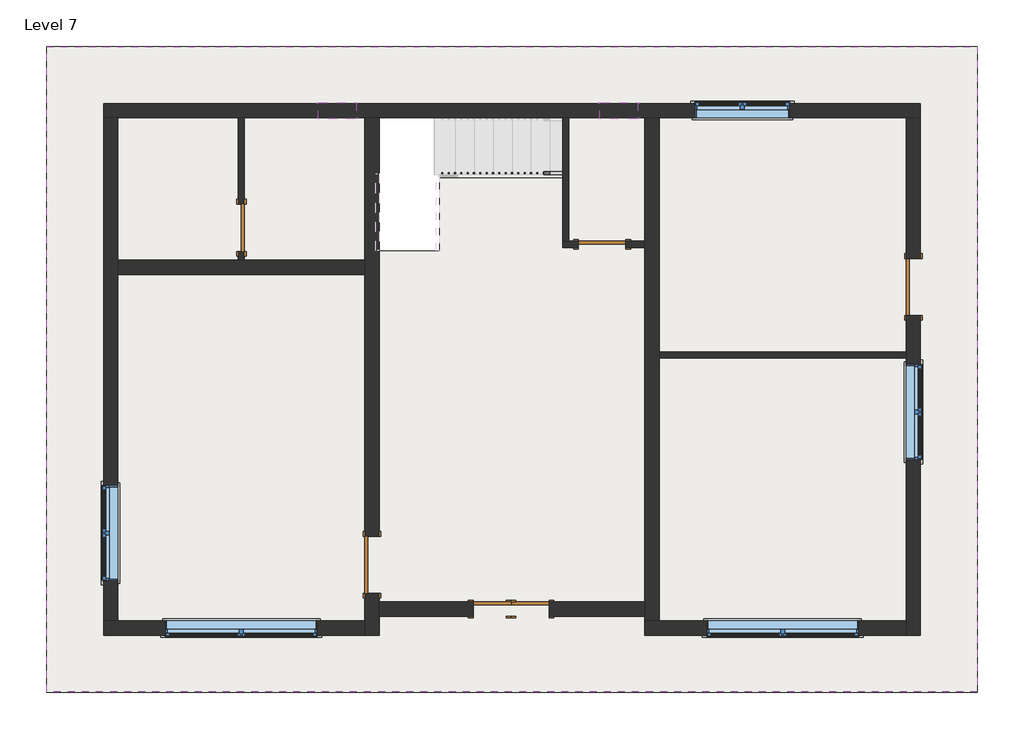
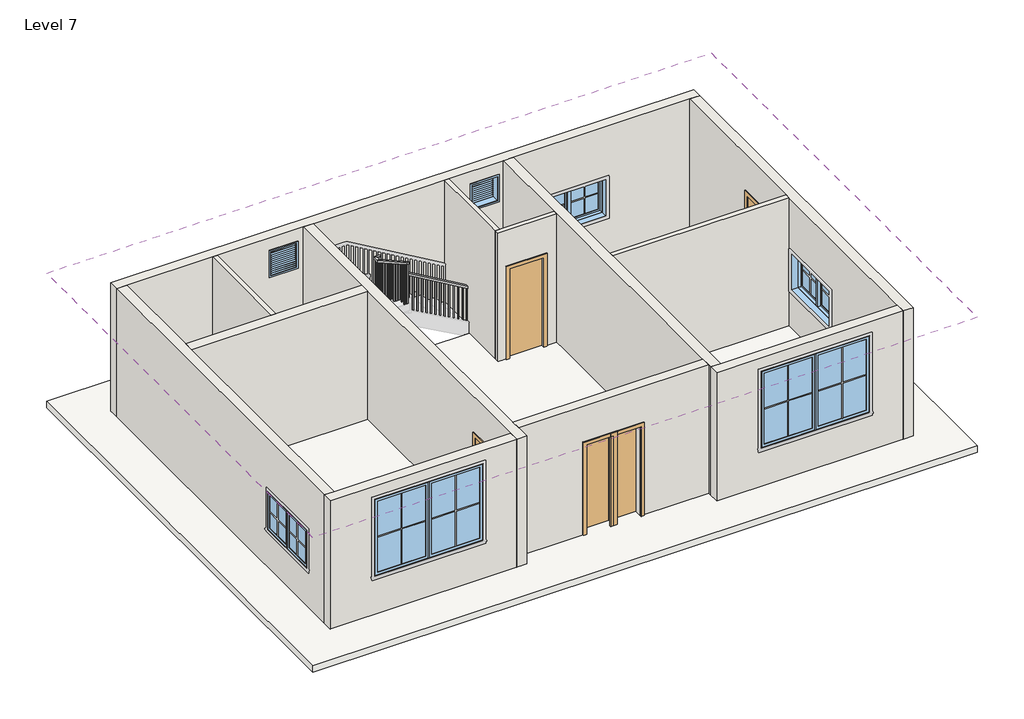
# One storey, part 1 of 2: 13 walls, 7 windows, 6 doors, 2 roofs, 1 railing.
"""IFC4 building model written with IfcOpenShell, lengths in millimetres."""

from ifc_helpers import new_model, si_unit, frame, origin, place, context, project, spatial, polyline, outline, extrude, faceted_brep, transform, mapped, element, save
from components import single_flush_door_2_4a3212df, single_flush_door_2_0d3b4037, door_270f2424, door_aa9e95e7, single_flush_door_3_a90ba1ad, window_casement_double_c1d95f0f, window_casement_double_9ae172a2, window_f2d8fef0

model = new_model("IFC4")

# Units and contexts
model_context = context("Model", 3, world=origin())
ifc_project = project(units=[si_unit("LENGTHUNIT", "METRE", prefix="MILLI")], contexts=[model_context])

# Site, building, storey
site = spatial("IfcSite", under=ifc_project)
building = spatial("IfcBuilding", under=site)
storey = spatial("IfcBuildingStorey", under=building, Name="Level 7", Elevation=19050.0)

# Doors
placement = place(None, origin())
single_flush_door_2_shape = single_flush_door_2_4a3212df(model_context)
element("IfcDoor", 1, ObjectType="Single-Flush : DOOR 2'", at=placement, inside=storey, context=model_context, shape_type="MappedRepresentation", body=[
    mapped(single_flush_door_2_shape, transform((-1572.7415084, -2604.3618005, 19050.0), x_axis=(-1.0, 0.0, 0.0), y_axis=(0.0, -1.0, 0.0), z_axis=(0.0, 0.0, 1.0))),
])
single_flush_door_2_2_shape = single_flush_door_2_0d3b4037(model_context)
element("IfcDoor", 2, ObjectType="Single-Flush : DOOR 2'", at=placement, inside=storey, context=model_context, shape_type="MappedRepresentation", body=[
    mapped(single_flush_door_2_2_shape, transform((-963.1415084, -2604.3618005, 19050.0), x_axis=(1.0, 0.0, 0.0), y_axis=(0.0, 1.0, 0.0), z_axis=(0.0, 0.0, 1.0))),
])
door_shape = door_270f2424(model_context)
element("IfcDoor", 3, ObjectType="Single-Flush : DOOR 2'6\"", at=placement, inside=storey, context=model_context, shape_type="MappedRepresentation", body=[
    mapped(door_shape, transform((-5598.6415084, 3517.0381995, 19050.0), x_axis=(0.0, -1.0, 0.0), y_axis=(1.0, 0.0, 0.0), z_axis=(0.0, 0.0, 1.0))),
])
door_2_shape = door_aa9e95e7(model_context)
element("IfcDoor", 4, ObjectType="Single-Flush : DOOR 2'6\"", at=placement, inside=storey, context=model_context, shape_type="MappedRepresentation", body=[
    mapped(door_2_shape, transform((192.5584916, 3250.3381995, 19050.0), x_axis=(-1.0, 0.0, 0.0), y_axis=(0.0, -1.0, 0.0), z_axis=(0.0, 0.0, 1.0))),
])
single_flush_door_3_shape = single_flush_door_3_a90ba1ad(model_context)
element("IfcDoor", 5, ObjectType="Single-Flush : DOOR 3'", at=placement, inside=storey, context=model_context, shape_type="MappedRepresentation", body=[
    mapped(single_flush_door_3_shape, transform((-3503.1415084, -1893.1618005, 19050.0), x_axis=(0.0, -1.0, 0.0), y_axis=(1.0, 0.0, 0.0), z_axis=(0.0, 0.0, 1.0))),
])
element("IfcDoor", 6, ObjectType="Single-Flush : DOOR 3'", at=placement, inside=storey, context=model_context, shape_type="MappedRepresentation", body=[
    mapped(single_flush_door_3_shape, transform((5183.6584916, 2564.5381995, 19050.0), x_axis=(0.0, -1.0, 0.0), y_axis=(1.0, 0.0, 0.0), z_axis=(0.0, 0.0, 1.0))),
])

# Railing
element("IfcRailing", 7, ObjectType="Handrail - Rectangular", at=placement, inside=storey, context=model_context, shape_type="SolidModel", body=[
    faceted_brep([(-442.4415084, 4368.3146777, 20133.7333333), (-442.4415084, 4368.3146777, 20074.9219871), (-442.4415084, 4419.1146777, 20074.9219871), (-442.4415084, 4419.1146777, 20133.7333333), (-2398.2415084, 4368.3146777, 21274.6166667), (-2449.0415084, 4368.3146777, 21245.4386538), (-2449.0415084, 4419.1146777, 21245.4386538), (-2398.2415084, 4419.1146777, 21274.6166667), (-2398.2415084, 4368.3146777, 21530.7202697), (-2449.0415084, 4368.3146777, 21479.9202697), (-2449.0415084, 4419.1146777, 21479.9202697), (-2398.2415084, 4419.1146777, 21530.7202697), (-2474.4415084, 4368.3146777, 21530.7202697), (-2474.4415084, 4368.3146777, 21479.9202697), (-2525.2415084, 4419.1146777, 21479.9202697), (-2525.2415084, 4419.1146777, 21530.7202697), (-2474.4415084, 4292.1146777, 21530.7202697), (-2474.4415084, 4278.9546266, 21479.9202697), (-2525.2415084, 4278.9546266, 21479.9202697), (-2525.2415084, 4292.1146777, 21530.7202697), (-2474.4415084, 3148.7383287, 22165.7333333), (-2525.2415084, 3148.7383287, 22165.7333333), (-2525.2415084, 3148.7383287, 22107.62445), (-2474.4415084, 3148.7383287, 22107.62445)], [[[0, 1, 2, 3]], [[1, 0, 4, 5]], [[2, 1, 5, 6]], [[3, 2, 6, 7]], [[0, 3, 7, 4]], [[5, 4, 8, 9]], [[6, 5, 9, 10]], [[7, 6, 10, 11]], [[4, 7, 11, 8]], [[9, 8, 12, 13]], [[10, 9, 13, 14]], [[11, 10, 14, 15]], [[8, 11, 15, 12]], [[13, 12, 16, 17]], [[14, 13, 17, 18]], [[15, 14, 18, 19]], [[12, 15, 19, 16]], [[20, 21, 22, 23]], [[17, 16, 20, 23]], [[18, 17, 23, 22]], [[19, 18, 22, 21]], [[16, 19, 21, 20]]]),
    extrude(outline(polyline([(3184.0396777, 22088.1754052), (3184.0396777, 21082.0), (3164.9896777, 21082.0), (3164.9896777, 22098.7554726), (3184.0396777, 22088.1754052)])), frame((-2509.3665084, 0.0, 0.0), z_axis=(1.0, 0.0, 0.0), x_axis=(0.0, 1.0, 0.0)), (0.0, 0.0, 1.0), 19.05),
    extrude(outline(polyline([(3285.6396777, 22031.7483789), (3285.6396777, 21082.0), (3266.5896777, 21082.0), (3266.5896777, 22042.3284463), (3285.6396777, 22031.7483789)])), frame((-2509.3665084, 0.0, 0.0), z_axis=(1.0, 0.0, 0.0), x_axis=(0.0, 1.0, 0.0)), (0.0, 0.0, 1.0), 19.05),
    extrude(outline(polyline([(3387.2396777, 21975.3213526), (3387.2396777, 21082.0), (3368.1896777, 21082.0), (3368.1896777, 21985.9014201), (3387.2396777, 21975.3213526)])), frame((-2509.3665084, 0.0, 0.0), z_axis=(1.0, 0.0, 0.0), x_axis=(0.0, 1.0, 0.0)), (0.0, 0.0, 1.0), 19.05),
    extrude(outline(polyline([(3488.8396777, 21918.8420718), (3488.8396777, 20912.6666667), (3469.7896777, 20912.6666667), (3469.7896777, 21929.4221392), (3488.8396777, 21918.8420718)])), frame((-2509.3665084, 0.0, 0.0), z_axis=(1.0, 0.0, 0.0), x_axis=(0.0, 1.0, 0.0)), (0.0, 0.0, 1.0), 19.05),
    extrude(outline(polyline([(3590.4396777, 21862.4150456), (3590.4396777, 20912.6666667), (3571.3896777, 20912.6666667), (3571.3896777, 21872.995113), (3590.4396777, 21862.4150456)])), frame((-2509.3665084, 0.0, 0.0), z_axis=(1.0, 0.0, 0.0), x_axis=(0.0, 1.0, 0.0)), (0.0, 0.0, 1.0), 19.05),
    extrude(outline(polyline([(3692.0396777, 21805.9880193), (3692.0396777, 20912.6666667), (3672.9896777, 20912.6666667), (3672.9896777, 21816.5680867), (3692.0396777, 21805.9880193)])), frame((-2509.3665084, 0.0, 0.0), z_axis=(1.0, 0.0, 0.0), x_axis=(0.0, 1.0, 0.0)), (0.0, 0.0, 1.0), 19.05),
    extrude(outline(polyline([(3793.6396777, 21749.5087385), (3793.6396777, 20743.3333333), (3774.5896777, 20743.3333333), (3774.5896777, 21760.0888059), (3793.6396777, 21749.5087385)])), frame((-2509.3665084, 0.0, 0.0), z_axis=(1.0, 0.0, 0.0), x_axis=(0.0, 1.0, 0.0)), (0.0, 0.0, 1.0), 19.05),
    extrude(outline(polyline([(3895.2396777, 21693.0817122), (3895.2396777, 20743.3333333), (3876.1896777, 20743.3333333), (3876.1896777, 21703.6617797), (3895.2396777, 21693.0817122)])), frame((-2509.3665084, 0.0, 0.0), z_axis=(1.0, 0.0, 0.0), x_axis=(0.0, 1.0, 0.0)), (0.0, 0.0, 1.0), 19.05),
    extrude(outline(polyline([(3996.8396777, 21636.654686), (3996.8396777, 20743.3333333), (3977.7896777, 20743.3333333), (3977.7896777, 21647.2347534), (3996.8396777, 21636.654686)])), frame((-2509.3665084, 0.0, 0.0), z_axis=(1.0, 0.0, 0.0), x_axis=(0.0, 1.0, 0.0)), (0.0, 0.0, 1.0), 19.05),
    extrude(outline(polyline([(4098.4396777, 21580.1754052), (4098.4396777, 20574.0), (4079.3896777, 20574.0), (4079.3896777, 21590.7554726), (4098.4396777, 21580.1754052)])), frame((-2509.3665084, 0.0, 0.0), z_axis=(1.0, 0.0, 0.0), x_axis=(0.0, 1.0, 0.0)), (0.0, 0.0, 1.0), 19.05),
    extrude(outline(polyline([(4200.0396777, 21523.7483789), (4200.0396777, 20574.0), (4180.9896777, 20574.0), (4180.9896777, 21534.3284463), (4200.0396777, 21523.7483789)])), frame((-2509.3665084, 0.0, 0.0), z_axis=(1.0, 0.0, 0.0), x_axis=(0.0, 1.0, 0.0)), (0.0, 0.0, 1.0), 19.05),
    extrude(outline(polyline([(4301.6396777, 21467.3213526), (4301.6396777, 20574.0), (4282.5896777, 20574.0), (4282.5896777, 21477.9014201), (4301.6396777, 21467.3213526)])), frame((-2509.3665084, 0.0, 0.0), z_axis=(1.0, 0.0, 0.0), x_axis=(0.0, 1.0, 0.0)), (0.0, 0.0, 1.0), 19.05),
    extrude(outline(polyline([(-2464.9165084, 4384.1896777), (-2483.9665084, 4384.1896777), (-2483.9665084, 4403.2396777), (-2464.9165084, 4403.2396777), (-2464.9165084, 4384.1896777)])), frame((0.0, 0.0, 20404.6666667), z_axis=(0.0, 0.0, 1.0), x_axis=(1.0, 0.0, 0.0)), (0.0, 0.0, 1.0), 1075.253603),
    extrude(outline(polyline([(21206.5449038, -2382.3665084), (20235.3333333, -2382.3665084), (20235.3333333, -2363.3165084), (21195.4324038, -2363.3165084), (21206.5449038, -2382.3665084)])), frame((0.0, 4384.1896777, 0.0), z_axis=(0.0, 1.0, 0.0), x_axis=(0.0, 0.0, 1.0)), (0.0, 0.0, 1.0), 19.05),
    extrude(outline(polyline([(21147.2782371, -2280.7665084), (20235.3333333, -2280.7665084), (20235.3333333, -2261.7165084), (21136.1657371, -2261.7165084), (21147.2782371, -2280.7665084)])), frame((0.0, 4384.1896777, 0.0), z_axis=(0.0, 1.0, 0.0), x_axis=(0.0, 0.0, 1.0)), (0.0, 0.0, 1.0), 19.05),
    extrude(outline(polyline([(21088.0115704, -2179.1665084), (20235.3333333, -2179.1665084), (20235.3333333, -2160.1165084), (21076.8990704, -2160.1165084), (21088.0115704, -2179.1665084)])), frame((0.0, 4384.1896777, 0.0), z_axis=(0.0, 1.0, 0.0), x_axis=(0.0, 0.0, 1.0)), (0.0, 0.0, 1.0), 19.05),
    extrude(outline(polyline([(21028.7449038, -2077.5665084), (20066.0, -2077.5665084), (20066.0, -2058.5165084), (21017.6324038, -2058.5165084), (21028.7449038, -2077.5665084)])), frame((0.0, 4384.1896777, 0.0), z_axis=(0.0, 1.0, 0.0), x_axis=(0.0, 0.0, 1.0)), (0.0, 0.0, 1.0), 19.05),
    extrude(outline(polyline([(20969.4782371, -1975.9665084), (20066.0, -1975.9665084), (20066.0, -1956.9165084), (20958.3657371, -1956.9165084), (20969.4782371, -1975.9665084)])), frame((0.0, 4384.1896777, 0.0), z_axis=(0.0, 1.0, 0.0), x_axis=(0.0, 0.0, 1.0)), (0.0, 0.0, 1.0), 19.05),
    extrude(outline(polyline([(20910.2115704, -1874.3665084), (20066.0, -1874.3665084), (20066.0, -1855.3165084), (20899.0990704, -1855.3165084), (20910.2115704, -1874.3665084)])), frame((0.0, 4384.1896777, 0.0), z_axis=(0.0, 1.0, 0.0), x_axis=(0.0, 0.0, 1.0)), (0.0, 0.0, 1.0), 19.05),
    extrude(outline(polyline([(20850.9449038, -1772.7665084), (19896.6666667, -1772.7665084), (19896.6666667, -1753.7165084), (20839.8324038, -1753.7165084), (20850.9449038, -1772.7665084)])), frame((0.0, 4384.1896777, 0.0), z_axis=(0.0, 1.0, 0.0), x_axis=(0.0, 0.0, 1.0)), (0.0, 0.0, 1.0), 19.05),
    extrude(outline(polyline([(20791.6782371, -1671.1665084), (19896.6666667, -1671.1665084), (19896.6666667, -1652.1165084), (20780.5657371, -1652.1165084), (20791.6782371, -1671.1665084)])), frame((0.0, 4384.1896777, 0.0), z_axis=(0.0, 1.0, 0.0), x_axis=(0.0, 0.0, 1.0)), (0.0, 0.0, 1.0), 19.05),
    extrude(outline(polyline([(20732.4115704, -1569.5665084), (19896.6666667, -1569.5665084), (19896.6666667, -1550.5165084), (20721.2990704, -1550.5165084), (20732.4115704, -1569.5665084)])), frame((0.0, 4384.1896777, 0.0), z_axis=(0.0, 1.0, 0.0), x_axis=(0.0, 0.0, 1.0)), (0.0, 0.0, 1.0), 19.05),
    extrude(outline(polyline([(20673.1449038, -1467.9665084), (19727.3333333, -1467.9665084), (19727.3333333, -1448.9165084), (20662.0324038, -1448.9165084), (20673.1449038, -1467.9665084)])), frame((0.0, 4384.1896777, 0.0), z_axis=(0.0, 1.0, 0.0), x_axis=(0.0, 0.0, 1.0)), (0.0, 0.0, 1.0), 19.05),
    extrude(outline(polyline([(20613.8782371, -1366.3665084), (19727.3333333, -1366.3665084), (19727.3333333, -1347.3165084), (20602.7657371, -1347.3165084), (20613.8782371, -1366.3665084)])), frame((0.0, 4384.1896777, 0.0), z_axis=(0.0, 1.0, 0.0), x_axis=(0.0, 0.0, 1.0)), (0.0, 0.0, 1.0), 19.05),
    extrude(outline(polyline([(20554.6115704, -1264.7665084), (19727.3333333, -1264.7665084), (19727.3333333, -1245.7165084), (20543.4990704, -1245.7165084), (20554.6115704, -1264.7665084)])), frame((0.0, 4384.1896777, 0.0), z_axis=(0.0, 1.0, 0.0), x_axis=(0.0, 0.0, 1.0)), (0.0, 0.0, 1.0), 19.05),
    extrude(outline(polyline([(20495.3449038, -1163.1665084), (19558.0, -1163.1665084), (19558.0, -1144.1165084), (20484.2324038, -1144.1165084), (20495.3449038, -1163.1665084)])), frame((0.0, 4384.1896777, 0.0), z_axis=(0.0, 1.0, 0.0), x_axis=(0.0, 0.0, 1.0)), (0.0, 0.0, 1.0), 19.05),
    extrude(outline(polyline([(20436.0782371, -1061.5665084), (19558.0, -1061.5665084), (19558.0, -1042.5165084), (20424.9657371, -1042.5165084), (20436.0782371, -1061.5665084)])), frame((0.0, 4384.1896777, 0.0), z_axis=(0.0, 1.0, 0.0), x_axis=(0.0, 0.0, 1.0)), (0.0, 0.0, 1.0), 19.05),
    extrude(outline(polyline([(20376.8115704, -959.9665084), (19558.0, -959.9665084), (19558.0, -940.9165084), (20365.6990704, -940.9165084), (20376.8115704, -959.9665084)])), frame((0.0, 4384.1896777, 0.0), z_axis=(0.0, 1.0, 0.0), x_axis=(0.0, 0.0, 1.0)), (0.0, 0.0, 1.0), 19.05),
    extrude(outline(polyline([(20317.5449038, -858.3665084), (19388.6666667, -858.3665084), (19388.6666667, -839.3165084), (20306.4324038, -839.3165084), (20317.5449038, -858.3665084)])), frame((0.0, 4384.1896777, 0.0), z_axis=(0.0, 1.0, 0.0), x_axis=(0.0, 0.0, 1.0)), (0.0, 0.0, 1.0), 19.05),
    extrude(outline(polyline([(20258.2782371, -756.7665084), (19388.6666667, -756.7665084), (19388.6666667, -737.7165084), (20247.1657371, -737.7165084), (20258.2782371, -756.7665084)])), frame((0.0, 4384.1896777, 0.0), z_axis=(0.0, 1.0, 0.0), x_axis=(0.0, 0.0, 1.0)), (0.0, 0.0, 1.0), 19.05),
    extrude(outline(polyline([(20199.0115704, -655.1665084), (19388.6666667, -655.1665084), (19388.6666667, -636.1165084), (20187.8990704, -636.1165084), (20199.0115704, -655.1665084)])), frame((0.0, 4384.1896777, 0.0), z_axis=(0.0, 1.0, 0.0), x_axis=(0.0, 0.0, 1.0)), (0.0, 0.0, 1.0), 19.05),
    extrude(outline(polyline([(20139.7449038, -553.5665084), (19219.3333333, -553.5665084), (19219.3333333, -534.5165084), (20128.6324038, -534.5165084), (20139.7449038, -553.5665084)])), frame((0.0, 4384.1896777, 0.0), z_axis=(0.0, 1.0, 0.0), x_axis=(0.0, 0.0, 1.0)), (0.0, 0.0, 1.0), 19.05),
    extrude(outline(polyline([(-2490.3165084, 4384.1896777), (-2509.3665084, 4384.1896777), (-2509.3665084, 4403.2396777), (-2490.3165084, 4403.2396777), (-2490.3165084, 4384.1896777)])), frame((0.0, 0.0, 20404.6666667), z_axis=(0.0, 0.0, 1.0), x_axis=(1.0, 0.0, 0.0)), (0.0, 0.0, 1.0), 1075.253603),
    extrude(outline(polyline([(3167.7883287, 22097.0443826), (3167.7883287, 21082.0), (3148.7383287, 21082.0), (3148.7383287, 22107.62445), (3167.7883287, 22097.0443826)])), frame((-2509.3665084, 0.0, 0.0), z_axis=(1.0, 0.0, 0.0), x_axis=(0.0, 1.0, 0.0)), (0.0, 0.0, 1.0), 19.05),
    extrude(outline(polyline([(20086.0344871, -461.4915084), (19219.3333333, -461.4915084), (19219.3333333, -442.4415084), (20074.9219871, -442.4415084), (20086.0344871, -461.4915084)])), frame((0.0, 4384.1896777, 0.0), z_axis=(0.0, 1.0, 0.0), x_axis=(0.0, 0.0, 1.0)), (0.0, 0.0, 1.0), 19.05),
])

# Roofs
element("IfcRoof", 8, ObjectType="ROOF 6\"", at=placement, inside=storey, context=model_context, shape_type="SweptSolid", body=[
    extrude(outline(polyline([(-8722.8415084, -3937.8618005), (-8722.8415084, 6425.3381995), (6212.3584916, 6425.3381995), (6212.3584916, -3937.8618005), (-8722.8415084, -3937.8618005)]), holes=[polyline([(-3439.6415084, 5333.1381995), (-3439.6415084, 3148.7383287), (-2423.6415084, 3148.7383287), (-2423.6415084, 4317.5146777), (-442.4415084, 4317.5146777), (-442.4415084, 5333.1381995), (-3439.6415084, 5333.1381995)])]), frame((0.0, 0.0, 18897.6), z_axis=(0.0, 0.0, 1.0), x_axis=(1.0, 0.0, 0.0)), (0.0, 0.0, 1.0), 152.4),
])
element("IfcRoof", 9, ObjectType="ROOF 6\"", at=placement, inside=storey, context=model_context, shape_type="SweptSolid", body=[
    extrude(outline(polyline([(-8722.8415084, -3937.8618005), (-8722.8415084, 6425.3381995), (6212.3584916, 6425.3381995), (6212.3584916, -3937.8618005), (-8722.8415084, -3937.8618005)]), holes=[polyline([(-3439.6415084, 5333.1381995), (-3439.6415084, 3148.7383287), (-2423.6415084, 3148.7383287), (-2423.6415084, 4317.5146777), (-442.4415084, 4317.5146777), (-442.4415084, 5333.1381995), (-3439.6415084, 5333.1381995)])]), frame((0.0, 0.0, 22098.0), z_axis=(0.0, 0.0, 1.0), x_axis=(1.0, 0.0, 0.0)), (0.0, 0.0, 1.0), 152.4),
])

# Walls
element("IfcWall", 10, ObjectType="WALL 4\"", at=placement, inside=storey, context=model_context, shape_type="SweptSolid", body=[
    extrude(outline(polyline([(3136.0381995, 21183.6), (3136.0381995, 19050.0), (2996.3381995, 19050.0), (2996.3381995, 22098.0), (5282.3381995, 22098.0), (5282.3381995, 19050.0), (3898.0381995, 19050.0), (3898.0381995, 21183.6), (3136.0381995, 21183.6)])), frame((-5649.4415084, 0.0, 0.0), z_axis=(1.0, 0.0, 0.0), x_axis=(0.0, 1.0, 0.0)), (0.0, 0.0, 1.0), 101.6),
])
element("IfcWall", 11, ObjectType="WALL 4\"", at=placement, inside=storey, context=model_context, shape_type="Brep", body=[
    faceted_brep([(-188.4415084, 3301.1381995, 21183.6), (-188.4415084, 3301.1381995, 19050.0), (-340.8415084, 3301.1381995, 19050.0), (-442.4415084, 3301.1381995, 19050.0), (-442.4415084, 3301.1381995, 22098.0), (-340.8415084, 3301.1381995, 22098.0), (878.3584916, 3301.1381995, 22098.0), (878.3584916, 3301.1381995, 19050.0), (573.5584916, 3301.1381995, 19050.0), (573.5584916, 3301.1381995, 21183.6), (-442.4415084, 3199.5381995, 19050.0), (-188.4415084, 3199.5381995, 19050.0), (-188.4415084, 3199.5381995, 21183.6), (573.5584916, 3199.5381995, 21183.6), (573.5584916, 3199.5381995, 19050.0), (878.3584916, 3199.5381995, 19050.0), (878.3584916, 3199.5381995, 22098.0), (-442.4415084, 3199.5381995, 22098.0)], [[[0, 1, 2, 3, 4, 5, 6, 7, 8, 9]], [[10, 11, 12, 13, 14, 15, 16, 17]], [[8, 7, 15, 14]], [[3, 2, 1, 11, 10]], [[7, 6, 16, 15]], [[4, 3, 10, 17]], [[12, 11, 1, 0]], [[13, 12, 0, 9]], [[14, 13, 9, 8]], [[6, 5, 4, 17, 16]]]),
])
element("IfcWall", 12, ObjectType="WALL 4\"", at=placement, inside=storey, context=model_context, shape_type="Brep", body=[
    faceted_brep([(-340.8415084, 3301.1381995, 19050.0), (-340.8415084, 5282.3381995, 19050.0), (-340.8415084, 5282.3381995, 22098.0), (-340.8415084, 3301.1381995, 22098.0), (-442.4415084, 3301.1381995, 19050.0), (-442.4415084, 3301.1381995, 22098.0), (-442.4415084, 4317.5146777, 22098.0), (-442.4415084, 5282.3381995, 22098.0), (-442.4415084, 5282.3381995, 19050.0)], [[[0, 1, 2, 3]], [[4, 5, 6, 7, 8]], [[1, 0, 4, 8]], [[0, 3, 5, 4]], [[2, 1, 8, 7]], [[3, 2, 7, 6, 5]]]),
])
element("IfcWall", 13, ObjectType="WALL 4\"", at=placement, inside=storey, context=model_context, shape_type="SweptSolid", body=[
    extrude(outline(polyline([(1106.9584916, 1523.1381995), (5069.3584916, 1523.1381995), (5069.3584916, 1421.5381995), (1106.9584916, 1421.5381995), (1106.9584916, 1523.1381995)])), frame((0.0, 0.0, 19050.0), z_axis=(0.0, 0.0, 1.0), x_axis=(1.0, 0.0, 0.0)), (0.0, 0.0, 1.0), 3048.0),
])
element("IfcWall", 14, ObjectType="WALL 9\"", at=placement, inside=storey, context=model_context, shape_type="Brep", body=[
    faceted_brep([(-7808.4415084, 5282.3381995, 19050.0), (-7579.8415084, 5282.3381995, 19050.0), (-5649.4415084, 5282.3381995, 19050.0), (-5547.8415084, 5282.3381995, 19050.0), (-3617.4415084, 5282.3381995, 19050.0), (-3388.8415084, 5282.3381995, 19050.0), (-442.4415084, 5282.3381995, 19050.0), (-340.8415084, 5282.3381995, 19050.0), (878.3584916, 5282.3381995, 19050.0), (1106.9584916, 5282.3381995, 19050.0), (5069.3584916, 5282.3381995, 19050.0), (5297.9584916, 5282.3381995, 19050.0), (5297.9584916, 5282.3381995, 22098.0), (5069.3584916, 5282.3381995, 22098.0), (1106.9584916, 5282.3381995, 22098.0), (878.3584916, 5282.3381995, 22098.0), (-340.8415084, 5282.3381995, 22098.0), (-442.4415084, 5282.3381995, 22098.0), (-3388.8415084, 5282.3381995, 22098.0), (-3617.4415084, 5282.3381995, 22098.0), (-5547.8415084, 5282.3381995, 22098.0), (-5649.4415084, 5282.3381995, 22098.0), (-7579.8415084, 5282.3381995, 22098.0), (-7808.4415084, 5282.3381995, 22098.0), (3202.4584916, 5282.3381995, 20878.8), (3202.4584916, 5282.3381995, 19964.4), (1678.4584916, 5282.3381995, 19964.4), (1678.4584916, 5282.3381995, 20878.8), (154.4584916, 5282.3381995, 21793.2), (764.0584916, 5282.3381995, 21793.2), (764.0584916, 5282.3381995, 21183.6), (154.4584916, 5282.3381995, 21183.6), (-3757.1415084, 5282.3381995, 21793.2), (-3757.1415084, 5282.3381995, 21183.6), (-4366.7415084, 5282.3381995, 21183.6), (-4366.7415084, 5282.3381995, 21793.2), (-7808.4415084, 5510.9381995, 19050.0), (-7808.4415084, 5510.9381995, 22098.0), (5297.9584916, 5510.9381995, 22098.0), (5297.9584916, 5510.9381995, 19050.0), (3202.4584916, 5510.9381995, 20878.8), (1678.4584916, 5510.9381995, 20878.8), (1678.4584916, 5510.9381995, 19964.4), (3202.4584916, 5510.9381995, 19964.4), (154.4584916, 5510.9381995, 21793.2), (154.4584916, 5510.9381995, 21183.6), (764.0584916, 5510.9381995, 21183.6), (764.0584916, 5510.9381995, 21793.2), (-3757.1415084, 5510.9381995, 21793.2), (-4366.7415084, 5510.9381995, 21793.2), (-4366.7415084, 5510.9381995, 21183.6), (-3757.1415084, 5510.9381995, 21183.6)], [[[0, 1, 2, 3, 4, 5, 6, 7, 8, 9, 10, 11, 12, 13, 14, 15, 16, 17, 18, 19, 20, 21, 22, 23], [24, 25, 26, 27], [28, 29, 30, 31], [32, 33, 34, 35]], [[36, 37, 38, 39], [40, 41, 42, 43], [44, 45, 46, 47], [48, 49, 50, 51]], [[11, 10, 9, 8, 7, 6, 5, 4, 3, 2, 1, 0, 36, 39]], [[23, 22, 21, 20, 19, 18, 17, 16, 15, 14, 13, 12, 38, 37]], [[12, 11, 39, 38]], [[0, 23, 37, 36]], [[25, 24, 40, 43]], [[26, 25, 43, 42]], [[27, 26, 42, 41]], [[24, 27, 41, 40]], [[45, 44, 28, 31]], [[46, 45, 31, 30]], [[47, 46, 30, 29]], [[44, 47, 29, 28]], [[33, 32, 48, 51]], [[34, 33, 51, 50]], [[35, 34, 50, 49]], [[32, 35, 49, 48]]]),
])
element("IfcWall", 15, ObjectType="WALL 9\"", at=placement, inside=storey, context=model_context, shape_type="Brep", body=[
    faceted_brep([(5069.3584916, 2107.3381995, 21183.6), (5069.3584916, 2107.3381995, 19050.0), (5069.3584916, 1523.1381995, 19050.0), (5069.3584916, 1421.5381995, 19050.0), (5069.3584916, -2794.8618005, 19050.0), (5069.3584916, -3023.4618005, 19050.0), (5069.3584916, -3023.4618005, 22098.0), (5069.3584916, -2794.8618005, 22098.0), (5069.3584916, 1421.5381995, 22098.0), (5069.3584916, 1523.1381995, 22098.0), (5069.3584916, 5282.3381995, 22098.0), (5069.3584916, 5282.3381995, 19050.0), (5069.3584916, 3021.7381995, 19050.0), (5069.3584916, 3021.7381995, 21183.6), (5069.3584916, -204.0618005, 20878.8), (5069.3584916, -204.0618005, 19964.4), (5069.3584916, 1319.9381995, 19964.4), (5069.3584916, 1319.9381995, 20878.8), (5297.9584916, -3023.4618005, 19050.0), (5297.9584916, 2107.3381995, 19050.0), (5297.9584916, 2107.3381995, 21183.6), (5297.9584916, 3021.7381995, 21183.6), (5297.9584916, 3021.7381995, 19050.0), (5297.9584916, 5282.3381995, 19050.0), (5297.9584916, 5282.3381995, 22098.0), (5297.9584916, -3023.4618005, 22098.0), (5297.9584916, -204.0618005, 20878.8), (5297.9584916, 1319.9381995, 20878.8), (5297.9584916, 1319.9381995, 19964.4), (5297.9584916, -204.0618005, 19964.4)], [[[0, 1, 2, 3, 4, 5, 6, 7, 8, 9, 10, 11, 12, 13], [14, 15, 16, 17]], [[18, 19, 20, 21, 22, 23, 24, 25], [26, 27, 28, 29]], [[12, 11, 23, 22]], [[5, 4, 3, 2, 1, 19, 18]], [[11, 10, 24, 23]], [[6, 5, 18, 25]], [[15, 14, 26, 29]], [[16, 15, 29, 28]], [[17, 16, 28, 27]], [[14, 17, 27, 26]], [[20, 19, 1, 0]], [[21, 20, 0, 13]], [[22, 21, 13, 12]], [[10, 9, 8, 7, 6, 25, 24]]]),
])
element("IfcWall", 16, ObjectType="WALL 9\"", at=placement, inside=storey, context=model_context, shape_type="Brep", body=[
    faceted_brep([(5069.3584916, -2794.8618005, 19050.0), (1106.9584916, -2794.8618005, 19050.0), (878.3584916, -2794.8618005, 19050.0), (878.3584916, -2794.8618005, 22098.0), (1106.9584916, -2794.8618005, 22098.0), (5069.3584916, -2794.8618005, 22098.0), (1868.9584916, -2794.8618005, 21793.2), (1868.9584916, -2794.8618005, 19964.4), (4307.3584916, -2794.8618005, 19964.4), (4307.3584916, -2794.8618005, 21793.2), (5069.3584916, -3023.4618005, 19050.0), (5069.3584916, -3023.4618005, 22098.0), (878.3584916, -3023.4618005, 22098.0), (878.3584916, -3023.4618005, 19050.0), (1868.9584916, -3023.4618005, 21793.2), (4307.3584916, -3023.4618005, 21793.2), (4307.3584916, -3023.4618005, 19964.4), (1868.9584916, -3023.4618005, 19964.4)], [[[0, 1, 2, 3, 4, 5], [6, 7, 8, 9]], [[10, 11, 12, 13], [14, 15, 16, 17]], [[2, 1, 0, 10, 13]], [[0, 5, 11, 10]], [[3, 2, 13, 12]], [[7, 6, 14, 17]], [[8, 7, 17, 16]], [[9, 8, 16, 15]], [[6, 9, 15, 14]], [[5, 4, 3, 12, 11]]]),
])
element("IfcWall", 17, ObjectType="WALL 9\"", at=placement, inside=storey, context=model_context, shape_type="Brep", body=[
    faceted_brep([(1106.9584916, -2794.8618005, 19050.0), (1106.9584916, 1421.5381995, 19050.0), (1106.9584916, 1523.1381995, 19050.0), (1106.9584916, 5282.3381995, 19050.0), (1106.9584916, 5282.3381995, 22098.0), (1106.9584916, 1523.1381995, 22098.0), (1106.9584916, 1421.5381995, 22098.0), (1106.9584916, -2794.8618005, 22098.0), (878.3584916, -2794.8618005, 19050.0), (878.3584916, -2794.8618005, 22098.0), (878.3584916, -2718.6618005, 22098.0), (878.3584916, -2490.0618005, 22098.0), (878.3584916, 3199.5381995, 22098.0), (878.3584916, 3301.1381995, 22098.0), (878.3584916, 5282.3381995, 22098.0), (878.3584916, 5282.3381995, 19050.0), (878.3584916, 3301.1381995, 19050.0), (878.3584916, 3199.5381995, 19050.0), (878.3584916, -2490.0618005, 19050.0), (878.3584916, -2718.6618005, 19050.0)], [[[0, 1, 2, 3, 4, 5, 6, 7]], [[8, 9, 10, 11, 12, 13, 14, 15, 16, 17, 18, 19]], [[3, 2, 1, 0, 8, 19, 18, 17, 16, 15]], [[0, 7, 9, 8]], [[4, 3, 15, 14]], [[7, 6, 5, 4, 14, 13, 12, 11, 10, 9]]]),
])
element("IfcWall", 18, ObjectType="WALL 9\"", at=placement, inside=storey, context=model_context, shape_type="SweptSolid", body=[
    extrude(outline(polyline([(19050.0, 878.3584916), (22098.0, 878.3584916), (22098.0, -3388.8415084), (19050.0, -3388.8415084), (19050.0, -1877.5415084), (21183.6, -1877.5415084), (21183.6, -658.3415084), (19050.0, -658.3415084), (19050.0, 878.3584916)])), frame((0.0, -2718.6618005, 0.0), z_axis=(0.0, 1.0, 0.0), x_axis=(0.0, 0.0, 1.0)), (0.0, 0.0, 1.0), 228.6),
])
element("IfcWall", 19, ObjectType="WALL 9\"", at=placement, inside=storey, context=model_context, shape_type="Brep", body=[
    faceted_brep([(-3388.8415084, -3023.4618005, 19050.0), (-3388.8415084, -2718.6618005, 19050.0), (-3388.8415084, -2490.0618005, 19050.0), (-3388.8415084, -2350.3618005, 19050.0), (-3388.8415084, -2350.3618005, 21183.6), (-3388.8415084, -1435.9618005, 21183.6), (-3388.8415084, -1435.9618005, 19050.0), (-3388.8415084, 5282.3381995, 19050.0), (-3388.8415084, 5282.3381995, 22098.0), (-3388.8415084, -2490.0618005, 22098.0), (-3388.8415084, -2718.6618005, 22098.0), (-3388.8415084, -3023.4618005, 22098.0), (-3617.4415084, -2350.3618005, 21183.6), (-3617.4415084, -2350.3618005, 19050.0), (-3617.4415084, -2794.8618005, 19050.0), (-3617.4415084, -3023.4618005, 19050.0), (-3617.4415084, -3023.4618005, 22098.0), (-3617.4415084, -2794.8618005, 22098.0), (-3617.4415084, 2767.7381995, 22098.0), (-3617.4415084, 2996.3381995, 22098.0), (-3617.4415084, 5282.3381995, 22098.0), (-3617.4415084, 5282.3381995, 19050.0), (-3617.4415084, 2996.3381995, 19050.0), (-3617.4415084, 2767.7381995, 19050.0), (-3617.4415084, -1435.9618005, 19050.0), (-3617.4415084, -1435.9618005, 21183.6)], [[[0, 1, 2, 3, 4, 5, 6, 7, 8, 9, 10, 11]], [[12, 13, 14, 15, 16, 17, 18, 19, 20, 21, 22, 23, 24, 25]], [[15, 14, 13, 3, 2, 1, 0]], [[24, 23, 22, 21, 7, 6]], [[11, 10, 9, 8, 20, 19, 18, 17, 16]], [[8, 7, 21, 20]], [[0, 11, 16, 15]], [[4, 3, 13, 12]], [[5, 4, 12, 25]], [[6, 5, 25, 24]]]),
])
element("IfcWall", 20, ObjectType="WALL 9\"", at=placement, inside=storey, context=model_context, shape_type="Brep", body=[
    faceted_brep([(-3617.4415084, -2794.8618005, 19050.0), (-7579.8415084, -2794.8618005, 19050.0), (-7808.4415084, -2794.8618005, 19050.0), (-7808.4415084, -2794.8618005, 22098.0), (-7579.8415084, -2794.8618005, 22098.0), (-3617.4415084, -2794.8618005, 22098.0), (-6817.8415084, -2794.8618005, 21793.2), (-6817.8415084, -2794.8618005, 19964.4), (-4379.4415084, -2794.8618005, 19964.4), (-4379.4415084, -2794.8618005, 21793.2), (-3617.4415084, -3023.4618005, 19050.0), (-3617.4415084, -3023.4618005, 22098.0), (-7808.4415084, -3023.4618005, 22098.0), (-7808.4415084, -3023.4618005, 19050.0), (-6817.8415084, -3023.4618005, 21793.2), (-4379.4415084, -3023.4618005, 21793.2), (-4379.4415084, -3023.4618005, 19964.4), (-6817.8415084, -3023.4618005, 19964.4)], [[[0, 1, 2, 3, 4, 5], [6, 7, 8, 9]], [[10, 11, 12, 13], [14, 15, 16, 17]], [[2, 1, 0, 10, 13]], [[0, 5, 11, 10]], [[3, 2, 13, 12]], [[7, 6, 14, 17]], [[8, 7, 17, 16]], [[9, 8, 16, 15]], [[6, 9, 15, 14]], [[5, 4, 3, 12, 11]]]),
])
element("IfcWall", 21, ObjectType="WALL 9\"", at=placement, inside=storey, context=model_context, shape_type="Brep", body=[
    faceted_brep([(-7579.8415084, -2794.8618005, 19050.0), (-7579.8415084, 2767.7381995, 19050.0), (-7579.8415084, 2996.3381995, 19050.0), (-7579.8415084, 5282.3381995, 19050.0), (-7579.8415084, 5282.3381995, 22098.0), (-7579.8415084, 2996.3381995, 22098.0), (-7579.8415084, 2767.7381995, 22098.0), (-7579.8415084, -2794.8618005, 22098.0), (-7579.8415084, -623.1618005, 20878.8), (-7579.8415084, -623.1618005, 19964.4), (-7579.8415084, -2147.1618005, 19964.4), (-7579.8415084, -2147.1618005, 20878.8), (-7808.4415084, -2794.8618005, 19050.0), (-7808.4415084, -2794.8618005, 22098.0), (-7808.4415084, 5282.3381995, 22098.0), (-7808.4415084, 5282.3381995, 19050.0), (-7808.4415084, -623.1618005, 20878.8), (-7808.4415084, -2147.1618005, 20878.8), (-7808.4415084, -2147.1618005, 19964.4), (-7808.4415084, -623.1618005, 19964.4)], [[[0, 1, 2, 3, 4, 5, 6, 7], [8, 9, 10, 11]], [[12, 13, 14, 15], [16, 17, 18, 19]], [[3, 2, 1, 0, 12, 15]], [[0, 7, 13, 12]], [[4, 3, 15, 14]], [[9, 8, 16, 19]], [[10, 9, 19, 18]], [[11, 10, 18, 17]], [[8, 11, 17, 16]], [[7, 6, 5, 4, 14, 13]]]),
])
element("IfcWall", 22, ObjectType="WALL 9\"", at=placement, inside=storey, context=model_context, shape_type="Brep", body=[
    faceted_brep([(-7579.8415084, 2767.7381995, 19050.0), (-3617.4415084, 2767.7381995, 19050.0), (-3617.4415084, 2767.7381995, 22098.0), (-7579.8415084, 2767.7381995, 22098.0), (-7579.8415084, 2996.3381995, 19050.0), (-7579.8415084, 2996.3381995, 22098.0), (-5649.4415084, 2996.3381995, 22098.0), (-5547.8415084, 2996.3381995, 22098.0), (-3617.4415084, 2996.3381995, 22098.0), (-3617.4415084, 2996.3381995, 19050.0), (-5547.8415084, 2996.3381995, 19050.0), (-5649.4415084, 2996.3381995, 19050.0)], [[[0, 1, 2, 3]], [[4, 5, 6, 7, 8, 9, 10, 11]], [[1, 0, 4, 11, 10, 9]], [[2, 1, 9, 8]], [[0, 3, 5, 4]], [[3, 2, 8, 7, 6, 5]]]),
])

# Windows
window_casement_double_shape = window_casement_double_c1d95f0f(model_context)
element("IfcWindow", 23, ObjectType="Window-Casement-Double", at=placement, inside=storey, context=model_context, shape_type="MappedRepresentation", body=[
    mapped(window_casement_double_shape, transform((-7694.1415084, -1385.1618005, 19050.0), x_axis=(0.0, 1.0, 0.0), y_axis=(-1.0, 0.0, 0.0), z_axis=(0.0, 0.0, 1.0))),
])
element("IfcWindow", 24, ObjectType="Window-Casement-Double", at=placement, inside=storey, context=model_context, shape_type="MappedRepresentation", body=[
    mapped(window_casement_double_shape, transform((5183.6584916, 557.9381995, 19050.0), x_axis=(0.0, -1.0, 0.0), y_axis=(1.0, 0.0, 0.0), z_axis=(0.0, 0.0, 1.0))),
])
element("IfcWindow", 25, ObjectType="Window-Casement-Double", at=placement, inside=storey, context=model_context, shape_type="MappedRepresentation", body=[
    mapped(window_casement_double_shape, transform((2440.4584916, 5396.6381995, 19050.0), x_axis=(1.0, 0.0, 0.0), y_axis=(0.0, 1.0, 0.0), z_axis=(0.0, 0.0, 1.0))),
])
window_casement_double_2_shape = window_casement_double_9ae172a2(model_context)
element("IfcWindow", 26, ObjectType="Window-Casement-Double", at=placement, inside=storey, context=model_context, shape_type="MappedRepresentation", body=[
    mapped(window_casement_double_2_shape, transform((-5598.6415084, -2909.1618005, 19050.0), x_axis=(-1.0, 0.0, 0.0), y_axis=(0.0, -1.0, 0.0), z_axis=(0.0, 0.0, 1.0))),
])
element("IfcWindow", 27, ObjectType="Window-Casement-Double", at=placement, inside=storey, context=model_context, shape_type="MappedRepresentation", body=[
    mapped(window_casement_double_2_shape, transform((3088.1584916, -2909.1618005, 19050.0), x_axis=(-1.0, 0.0, 0.0), y_axis=(0.0, -1.0, 0.0), z_axis=(0.0, 0.0, 1.0))),
])
window_shape = window_f2d8fef0(model_context)
element("IfcWindow", 28, ObjectType="Window-Louvers : 24\" x 24\"", at=placement, inside=storey, context=model_context, shape_type="MappedRepresentation", body=[
    mapped(window_shape, transform((459.2584916, 5402.9881995, 20269.2), x_axis=(1.0, 0.0, 0.0), y_axis=(0.0, 1.0, 0.0), z_axis=(0.0, 0.0, 1.0))),
])
element("IfcWindow", 29, ObjectType="Window-Louvers : 24\" x 24\"", at=placement, inside=storey, context=model_context, shape_type="MappedRepresentation", body=[
    mapped(window_shape, transform((-4061.9415084, 5390.2881995, 20269.2), x_axis=(-1.0, 0.0, 0.0), y_axis=(0.0, -1.0, 0.0), z_axis=(0.0, 0.0, 1.0))),
])

save(model, "model.ifc")

# Revit data of these elements
# Type "Single-Flush : DOOR 2'"
#   Type Mark = "10"
#   Construction Type Id = "MDOOR"
#   Assembly Code = "C1020"
#   Analytic Construction = "Metal"
#   Thickness = 0' - 2"
#   Heat Transfer Coefficient (U) = 0.651978 BTU/(h·ft²·°F)
#   Height = 7' - 0"
#   Trim Projection Ext = 0' - 1"
#   Trim Projection Int = 0' - 1"
#   Trim Width = 0' - 3"
#   Width = 2' - 0"
#   Define Thermal Properties by = 1
#   Door Material = Door - Panel
#   Frame Material = Door - Frame
#   Visual Light Transmittance = 0
#   Solar Heat Gain Coefficient = 0
#   Function = (empty or 0)
#   Wall Closure = (empty or 0)
# Type "Single-Flush : DOOR 2'6\""
#   Type Mark = "9"
#   Construction Type Id = "MDOOR"
#   Assembly Code = "C1020"
#   Analytic Construction = "Metal"
#   Thickness = 0' - 2"
#   Heat Transfer Coefficient (U) = 0.651978 BTU/(h·ft²·°F)
#   Height = 7' - 0"
#   Trim Projection Ext = 0' - 1"
#   Trim Projection Int = 0' - 1"
#   Trim Width = 0' - 3"
#   Width = 2' - 6"
#   Define Thermal Properties by = 1
#   Door Material = Door - Panel
#   Frame Material = Door - Frame
#   Visual Light Transmittance = 0
#   Solar Heat Gain Coefficient = 0
#   Function = (empty or 0)
#   Wall Closure = (empty or 0)
# Type "Single-Flush : DOOR 3'"
#   Type Mark = "8"
#   Construction Type Id = "MDOOR"
#   Assembly Code = "C1020"
#   Analytic Construction = "Metal"
#   Thickness = 0' - 2"
#   Heat Transfer Coefficient (U) = 0.651978 BTU/(h·ft²·°F)
#   Height = 7' - 0"
#   Trim Projection Ext = 0' - 1"
#   Trim Projection Int = 0' - 1"
#   Trim Width = 0' - 3"
#   Width = 3' - 0"
#   Define Thermal Properties by = 1
#   Door Material = Door - Panel
#   Frame Material = Door - Frame
#   Visual Light Transmittance = 0
#   Solar Heat Gain Coefficient = 0
#   Function = (empty or 0)
#   Wall Closure = (empty or 0)
# Type "Handrail - Rectangular"
#   Assembly Code = "C2010400"
#   built-in parameter 1008612 = 0.0416667 (stored number, unit not read)
#   built-in parameter 1008611 = 0.0416667 (stored number, unit not read)
#   built-in parameter 1008609 = 0.333333 (stored number, unit not read)
#   built-in parameter 1008604 = 0.166667 (stored number, unit not read)
#   built-in parameter 1008603 = 0.166667 (stored number, unit not read)
#   Railing Height = 3' - 0"
#   built-in parameter 1008630 = 2
#   built-in parameter 1008610 = 2
#   built-in parameter 1008618 = Baluster - Square : 3/4"
# Type "ROOF 6\""
#   Assembly Code = "B1020"
#   Layers, outside or top first: 0' - 6" no material (function 1)
# Type "WALL 4\""
#   Assembly Code = "B2010"
#   Layers, outside or top first: 0' - 4" no material (function 1)
# Type "WALL 9\""
#   Assembly Code = "B2010"
#   Layers, outside or top first: 0' - 9" no material (function 1)
# Type "Window-Casement-Double"
#   Type Mark = "18"
#   Fire Rating = "0.5h"
#   Assembly Code = "B2020100"
#   Analytic Construction = "Double glazing - domestic"
#   Frame Extension [instance default] = 0' - 0 1/4"
#   Window Inset [instance default] = 0' - 0"
#   Wall Thickness [instance default] = 0' - 6"
#   Interior Wall Closure [instance default] = 0' - 2 1/4"
#   Half Width = 2' - 6"
#   Visual Light Transmittance = 0.81
#   Thermal Resistance (R) = 1.8146 (h·ft²·°F)/BTU
#   Solar Heat Gain Coefficient = 0.76
#   Rough Width = 5' - 0 1/2"
#   Rough Height = 3' - 0 1/2"
#   Height = 3' - 0"
#   Heat Transfer Coefficient (U) = 0.5511 BTU/(h·ft²·°F)
#   Exterior Wall Closure [instance default] = 0' - 1 1/4"
#   Extension Jamb [instance default] = 0' - 2 1/4"
#   Default Sill Height = 3' - 0"
#   Width = 5' - 0"
#   Muntin Visibility = yes
#   Interior Trim Visibility [instance default] = yes
#   Exterior Trim Visibility [instance default] = yes
#   Extension Jamb Visibility [instance default] = yes
#   Interior Trim Material = Wood - Stained
#   Muntin Pattern = Muntin Pattern_2x2 : Muntin Pattern_2x2
#   Interior Trim = Trim-Window-Interior-Flat : Picture Frame
#   Interior Frame Material = Wood - Stained
#   Glass Panel Material = Glass
#   Exterior Trim Material = Clad - White
#   Exterior Trim = Trim-Window-Exterior-Flat : with Sill
#   Exterior Frame Material = Clad - White
#   Wall Closure = (empty or 0)
# Type "Window-Casement-Double"
#   Type Mark = "19"
#   Fire Rating = "0.5h"
#   Assembly Code = "B2020100"
#   Analytic Construction = "Double glazing - domestic"
#   Frame Extension [instance default] = 0' - 0 1/4"
#   Window Inset [instance default] = 0' - 0"
#   Wall Thickness [instance default] = 0' - 6"
#   Interior Wall Closure [instance default] = 0' - 2 1/4"
#   Half Width = 4' - 0"
#   Visual Light Transmittance = 0.81
#   Thermal Resistance (R) = 1.8146 (h·ft²·°F)/BTU
#   Solar Heat Gain Coefficient = 0.76
#   Rough Width = 8' - 0 1/2"
#   Rough Height = 6' - 0 1/2"
#   Height = 6' - 0"
#   Heat Transfer Coefficient (U) = 0.5511 BTU/(h·ft²·°F)
#   Exterior Wall Closure [instance default] = 0' - 1 1/4"
#   Extension Jamb [instance default] = 0' - 2 1/4"
#   Default Sill Height = 3' - 0"
#   Width = 8' - 0"
#   Muntin Visibility = yes
#   Interior Trim Visibility [instance default] = yes
#   Exterior Trim Visibility [instance default] = yes
#   Extension Jamb Visibility [instance default] = yes
#   Interior Trim Material = Wood - Stained
#   Muntin Pattern = Muntin Pattern_2x2 : Muntin Pattern_2x2
#   Interior Trim = Trim-Window-Interior-Flat : Picture Frame
#   Interior Frame Material = Wood - Stained
#   Glass Panel Material = Glass
#   Exterior Trim Material = Clad - White
#   Exterior Trim = Trim-Window-Exterior-Flat : with Sill
#   Exterior Frame Material = Clad - White
#   Wall Closure = (empty or 0)
# Type "Window-Louvers : 24\" x 24\""
#   Type Mark = "20"
#   Construction Type Id = "GSP4R"
#   Assembly Code = "B20"
#   Analytic Construction = "1/8 in Pilkington single glazing"
#   Visual Light Transmittance = 0.9
#   Thermal Resistance (R) = 1.53941 (h·ft²·°F)/BTU
#   Solar Heat Gain Coefficient = 0.78
#   Max Height = 1' - 11.74264"
#   Height = 2' - 0"
#   Heat Transfer Coefficient (U) = 0.6496 BTU/(h·ft²·°F)
#   Blade Width [instance default] = 1' - 10 1/2"
#   Blade Vertical Thickness = 0' - 0.35355"
#   Blade Thickness = 0' - 0 1/4"
#   Blade Spacing = 0' - 1 1/2"
#   Blade Height = 0' - 1.85355"
#   Blade Depth = 0' - 3"
#   Blade Angle = 45.00°
#   Default Sill Height = 3' - 0"
#   Trim Projection_Exterior = 0' - 0 1/2"
#   Trim Projection_Interior = 0' - 0 1/2"
#   Trim Width_Exterior = 0' - 1 1/2"
#   Trim Width_Interior = 0' - 1 1/2"
#   Width = 2' - 0"
#   Max Blade Count = 12
#   Define Thermal Properties by = 1
#   Blade Count = 12
#   Frame Material = Birch
#   Louver Material = Birch
#   Trim Exterior Material = Birch
#   Trim Interior Material = Birch
#   Wall Closure = (empty or 0)
# Elements 1, 2 (IfcDoor, "Single-Flush : DOOR 2'")
#   Phase Created = New Construction
#   Materials on its faces: "Door - Frame", "Door - Panel"
# Elements 3, 4 (IfcDoor, "Single-Flush : DOOR 2'6\"")
#   Phase Created = New Construction
#   Materials on its faces: "Door - Frame", "Door - Panel"
# Elements 5, 6 (IfcDoor, "Single-Flush : DOOR 3'")
#   Phase Created = New Construction
#   Materials on its faces: "Door - Frame", "Door - Panel"
# Element 7 (IfcRailing, "Handrail - Rectangular")
#   Phase Created = New Construction
# Element 8 (IfcRoof, "ROOF 6\"")
#   built-in parameter 1001705 = 62.5 (stored number, unit not read)
#   built-in parameter 1001701 = -0.5 (stored number, unit not read)
#   built-in parameter 1001710 = 33615
#   Phase Created = New Construction
#   Materials on its faces: "Door - Frame", "Default Roof", "Wood - Stained"
# Element 9 (IfcRoof, "ROOF 6\"")
#   built-in parameter 1001705 = 73 (stored number, unit not read)
#   built-in parameter 1001701 = 10 (stored number, unit not read)
#   built-in parameter 1001710 = 33615
#   Phase Created = New Construction
#   Materials on its faces: "Door - Frame", "Default Roof", "Wood - Stained"
# Elements 10, 13 (IfcWall, "WALL 4\"")
#   Top Offset = 0' - 0"
#   Base Offset = 0' - 0"
#   Unconnected Height = 10' - 0"
#   wall height = 10' - 0"
#   Phase Created = New Construction
#   Base Constraint = Level 7
#   Materials on its faces: "Default Wall"
# Elements 11, 12 (IfcWall, "WALL 4\"")
#   Top Offset = 0' - 0"
#   Base Offset = 0' - 0"
#   Unconnected Height = 10' - 0"
#   wall height = 10' - 0"
#   Phase Created = New Construction
#   Base Constraint = Level 7
#   Materials on its faces: "Default Wall", "Door - Frame"
# Element 14 (IfcWall, "WALL 9\"")
#   Top Offset = 0' - 0"
#   Base Offset = 0' - 0"
#   Unconnected Height = 10' - 0"
#   wall height = 10' - 0"
#   Phase Created = New Construction
#   Base Constraint = Level 7
#   Materials on its faces: "Default Wall", "Parking Stripe", "Door - Frame"
# Elements 15, 16, 17, 18, 20, 21 (IfcWall, "WALL 9\"")
#   Top Offset = 0' - 0"
#   Base Offset = 0' - 0"
#   Unconnected Height = 10' - 0"
#   wall height = 10' - 0"
#   Phase Created = New Construction
#   Base Constraint = Level 7
#   Materials on its faces: "Default Wall", "Parking Stripe"
# Element 19 (IfcWall, "WALL 9\"")
#   Top Offset = 0' - 0"
#   Base Offset = 0' - 0"
#   Unconnected Height = 10' - 0"
#   wall height = 10' - 0"
#   Phase Created = New Construction
#   Base Constraint = Level 7
#   Materials on its faces: "Default Wall", "Door - Frame", "Parking Stripe"
# Element 22 (IfcWall, "WALL 9\"")
#   Top Offset = 0' - 0"
#   Base Offset = 0' - 0"
#   Unconnected Height = 10' - 0"
#   wall height = 10' - 0"
#   Phase Created = New Construction
#   Base Constraint = Level 7
#   Materials on its faces: "Default Wall"
# Element 23 (IfcWindow, "Window-Casement-Double")
#   Mark = "43"
#   Window Inset = 0' - 0"
#   Interior Wall Closure = 0' - 2 1/4"
#   Frame Extension = 0' - 0 1/4"
#   Exterior Wall Closure = 0' - 1 1/4"
#   Interior Trim Visibility = yes
#   Exterior Trim Visibility = yes
#   Phase Created = New Construction
#   Materials on its faces: "Wood - Stained", "Glass", "Clad - White"
# Element 24 (IfcWindow, "Window-Casement-Double")
#   Mark = "44"
#   Window Inset = 0' - 0"
#   Interior Wall Closure = 0' - 2 1/4"
#   Frame Extension = 0' - 0 1/4"
#   Exterior Wall Closure = 0' - 1 1/4"
#   Interior Trim Visibility = yes
#   Exterior Trim Visibility = yes
#   Phase Created = New Construction
#   Materials on its faces: "Wood - Stained", "Glass", "Clad - White"
# Element 25 (IfcWindow, "Window-Casement-Double")
#   Mark = "45"
#   Window Inset = 0' - 0"
#   Interior Wall Closure = 0' - 2 1/4"
#   Frame Extension = 0' - 0 1/4"
#   Exterior Wall Closure = 0' - 1 1/4"
#   Interior Trim Visibility = yes
#   Exterior Trim Visibility = yes
#   Phase Created = New Construction
#   Materials on its faces: "Wood - Stained", "Glass", "Clad - White"
# Element 26 (IfcWindow, "Window-Casement-Double")
#   Mark = "46"
#   Window Inset = 0' - 0"
#   Interior Wall Closure = 0' - 2 1/4"
#   Frame Extension = 0' - 0 1/4"
#   Exterior Wall Closure = 0' - 1 1/4"
#   Interior Trim Visibility = yes
#   Exterior Trim Visibility = yes
#   Phase Created = New Construction
#   Materials on its faces: "Wood - Stained", "Glass", "Clad - White"
# Element 27 (IfcWindow, "Window-Casement-Double")
#   Mark = "47"
#   Window Inset = 0' - 0"
#   Interior Wall Closure = 0' - 2 1/4"
#   Frame Extension = 0' - 0 1/4"
#   Exterior Wall Closure = 0' - 1 1/4"
#   Interior Trim Visibility = yes
#   Exterior Trim Visibility = yes
#   Phase Created = New Construction
#   Materials on its faces: "Wood - Stained", "Glass", "Clad - White"
# Element 28 (IfcWindow, "Window-Louvers : 24\" x 24\"")
#   Mark = "48"
#   Blade Width = 1' - 10 1/2"
#   Phase Created = New Construction
#   Materials on its faces: "Birch"
# Element 29 (IfcWindow, "Window-Louvers : 24\" x 24\"")
#   Mark = "49"
#   Blade Width = 1' - 10 1/2"
#   Phase Created = New Construction
#   Materials on its faces: "Birch"
# Materials
#   "Door - Panel": class "Wood", colour RGB 210 159 95, transparency 0, Cost = 0
#   "Door - Frame": colour RGB 118 70 51, transparency 0, Cost = 0
#   "Wood - Stained": class "Wood", colour RGB 224 178 126, transparency 0, Cost = 0
#   "Glass": class "Glass", colour RGB 0 128 192, transparency 0.75, Description = "Soda Lime Glass", Cost = 0
#   "Clad - White": class "Wood", colour RGB 242 242 238, transparency 0, Cost = 0
#   "Birch": class "Wood", colour RGB 224 178 126, transparency 0, Description = "Betula Alleghaniensis", Cost = 0
#   "Default Roof": colour RGB 88 101 114, transparency 0, Cost = 0
#   "Default Wall": colour RGB 128 128 128, transparency 0, Cost = 0
#   "Parking Stripe": class "Paint", colour RGB 250 250 91, transparency 0, Cost = 0
